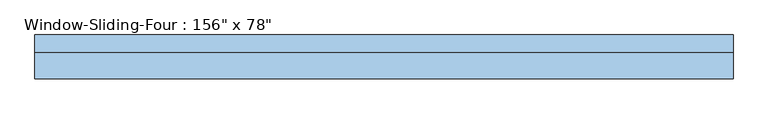
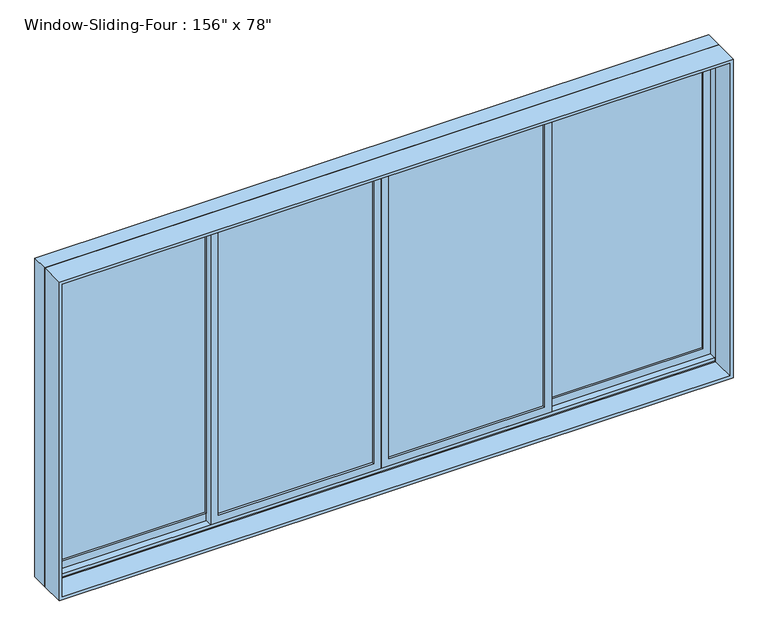
"""IFC4 building model written with IfcOpenShell, lengths in millimetres: window geometry."""

from ifc_helpers import new_model, si_unit, frame, origin, place, context, project, spatial, polyline, outline, extrude, faceted_brep, source, transform, mapped, element, save


def window_8ea0b4a1(model_context):
    return source(origin(), model_context, "Body", "SolidModel", [
        extrude(outline(polyline([(933.45, -1962.15), (933.45, -958.85), (2876.55, -958.85), (2876.55, -1962.15), (933.45, -1962.15)]), holes=[polyline([(2832.1, -1003.3), (996.95, -1003.3), (996.95, -1917.7), (2832.1, -1917.7), (2832.1, -1003.3)])]), frame((0.0, 78.74, 0.0), z_axis=(0.0, 1.0, 0.0), x_axis=(0.0, 0.0, 1.0)), (0.0, 0.0, 1.0), 44.45),
        extrude(outline(polyline([(-1003.3, 110.49), (-1003.3, 104.14), (-1917.7, 104.14), (-1917.7, 110.49), (-1003.3, 110.49)])), frame((0.0, 0.0, 996.95), z_axis=(0.0, 0.0, 1.0), x_axis=(1.0, 0.0, 0.0)), (0.0, 0.0, 1.0), 1835.15),
        extrude(outline(polyline([(-1003.3, 97.79), (-1003.3, 91.44), (-1917.7, 91.44), (-1917.7, 97.79), (-1003.3, 97.79)])), frame((0.0, 0.0, 996.95), z_axis=(0.0, 0.0, 1.0), x_axis=(1.0, 0.0, 0.0)), (0.0, 0.0, 1.0), 1835.15),
        extrude(outline(polyline([(-44.45, 66.04), (-44.45, 59.69), (-958.85, 59.69), (-958.85, 66.04), (-44.45, 66.04)])), frame((0.0, 0.0, 996.95), z_axis=(0.0, 0.0, 1.0), x_axis=(1.0, 0.0, 0.0)), (0.0, 0.0, 1.0), 1835.15),
        extrude(outline(polyline([(-44.45, 53.34), (-44.45, 46.99), (-958.85, 46.99), (-958.85, 53.34), (-44.45, 53.34)])), frame((0.0, 0.0, 996.95), z_axis=(0.0, 0.0, 1.0), x_axis=(1.0, 0.0, 0.0)), (0.0, 0.0, 1.0), 1835.15),
        extrude(outline(polyline([(2895.6, -1981.2), (914.4, -1981.2), (914.4, 1981.2), (2895.6, 1981.2), (2895.6, -1981.2)]), holes=[polyline([(2876.55, 1962.15), (933.45, 1962.15), (933.45, -1962.15), (2876.55, -1962.15), (2876.55, 1962.15)])]), frame((0.0, -118.11, 0.0), z_axis=(0.0, 1.0, 0.0), x_axis=(0.0, 0.0, 1.0)), (0.0, 0.0, 1.0), 146.05),
        extrude(outline(polyline([(952.5, 1003.3), (2876.55, 1003.3), (2876.55, 0.0), (952.5, 0.0), (952.5, 1003.3)]), holes=[polyline([(996.95, 44.45), (2832.1, 44.45), (2832.1, 958.85), (996.95, 958.85), (996.95, 44.45)])]), frame((0.0, 34.29, 0.0), z_axis=(0.0, 1.0, 0.0), x_axis=(0.0, 0.0, 1.0)), (0.0, 0.0, 1.0), 44.45),
        extrude(outline(polyline([(2876.55, -1003.3), (952.5, -1003.3), (952.5, 0.0), (2876.55, 0.0), (2876.55, -1003.3)]), holes=[polyline([(2832.1, -44.45), (996.95, -44.45), (996.95, -958.85), (2832.1, -958.85), (2832.1, -44.45)])]), frame((0.0, 34.29, 0.0), z_axis=(0.0, 1.0, 0.0), x_axis=(0.0, 0.0, 1.0)), (0.0, 0.0, 1.0), 44.45),
        extrude(outline(polyline([(958.85, 66.04), (958.85, 59.69), (44.45, 59.69), (44.45, 66.04), (958.85, 66.04)])), frame((0.0, 0.0, 996.95), z_axis=(0.0, 0.0, 1.0), x_axis=(1.0, 0.0, 0.0)), (0.0, 0.0, 1.0), 1835.15),
        extrude(outline(polyline([(958.85, 53.34), (958.85, 46.99), (44.45, 46.99), (44.45, 53.34), (958.85, 53.34)])), frame((0.0, 0.0, 996.95), z_axis=(0.0, 0.0, 1.0), x_axis=(1.0, 0.0, 0.0)), (0.0, 0.0, 1.0), 1835.15),
        extrude(outline(polyline([(1917.7, 110.49), (1917.7, 104.14), (1003.3, 104.14), (1003.3, 110.49), (1917.7, 110.49)])), frame((0.0, 0.0, 996.95), z_axis=(0.0, 0.0, 1.0), x_axis=(1.0, 0.0, 0.0)), (0.0, 0.0, 1.0), 1835.15),
        extrude(outline(polyline([(1917.7, 97.4725303), (1917.7, 91.44), (1003.3, 91.44), (1003.3, 97.4725303), (1917.7, 97.4725303)])), frame((0.0, 0.0, 996.95), z_axis=(0.0, 0.0, 1.0), x_axis=(1.0, 0.0, 0.0)), (0.0, 0.0, 1.0), 1835.15),
        extrude(outline(polyline([(933.45, 1962.15), (2876.55, 1962.15), (2876.55, 958.85), (933.45, 958.85), (933.45, 1962.15)]), holes=[polyline([(2832.1, 1003.3), (2832.1, 1917.7), (996.95, 1917.7), (996.95, 1003.3), (2832.1, 1003.3)])]), frame((0.0, 78.74, 0.0), z_axis=(0.0, 1.0, 0.0), x_axis=(0.0, 0.0, 1.0)), (0.0, 0.0, 1.0), 44.45),
        faceted_brep([(-1981.2, 27.94, 914.4), (-1981.2, 129.54, 914.4), (1981.2, 129.54, 914.4), (1981.2, 27.94, 914.4), (-1940.2778905, 129.54, 2854.6778905), (-1940.2778905, 123.19, 2854.6778905), (-1940.2778905, 123.19, 933.45), (-1940.2778905, 129.54, 933.45), (1940.2778905, 123.19, 2854.6778905), (1940.2778905, 123.19, 933.45), (1962.15, 123.19, 933.45), (1962.15, 123.19, 2876.55), (-1962.15, 123.19, 2876.55), (-1962.15, 123.19, 933.45), (-1962.15, 27.94, 2876.55), (-1962.15, 27.94, 933.45), (-1962.15, 34.29, 933.45), (-1962.15, 34.29, 952.5), (-1962.15, 78.74, 952.5), (-1962.15, 78.74, 933.45), (1981.2, 27.94, 2895.6), (-1981.2, 27.94, 2895.6), (1962.15, 27.94, 2876.55), (1962.15, 27.94, 933.45), (-1981.2, 129.54, 2895.6), (1981.2, 129.54, 2895.6), (1940.2778905, 129.54, 933.45), (1940.2778905, 129.54, 2854.6778905), (1962.15, 78.74, 933.45), (1962.15, 78.74, 952.5), (1962.15, 34.29, 952.5), (1962.15, 34.29, 933.45)], [[[0, 1, 2, 3]], [[4, 5, 6, 7]], [[5, 8, 9, 10, 11, 12, 13, 6]], [[12, 14, 15, 16, 17, 18, 19, 13]], [[0, 3, 20, 21], [22, 23, 15, 14]], [[24, 1, 0, 21]], [[2, 1, 24, 25], [4, 7, 26, 27]], [[5, 4, 27, 8]], [[12, 11, 22, 14]], [[21, 20, 25, 24]], [[8, 27, 26, 9]], [[22, 11, 10, 28, 29, 30, 31, 23]], [[20, 3, 2, 25]], [[26, 7, 6, 13, 19, 28, 10, 9]], [[28, 19, 18, 29]], [[29, 18, 17, 30]], [[30, 17, 16, 31]], [[15, 23, 31, 16]]]),
    ])


if __name__ == "__main__":
    model = new_model("IFC4")
    model_context = context("Model", 3, world=origin())
    ifc_project = project(units=[si_unit("LENGTHUNIT", "METRE", prefix="MILLI")], contexts=[model_context])
    site = spatial("IfcSite", under=ifc_project)
    building = spatial("IfcBuilding", under=site)
    placement = place(None, origin())
    window_shape = window_8ea0b4a1(model_context)
    element("IfcWindow", 1, ObjectType="Window-Sliding-Four : 156\" x 78\"", at=placement, inside=building, context=model_context, shape_type="MappedRepresentation", body=[
        mapped(window_shape, transform((0.0, 0.0, 0.0), x_axis=(1.0, 0.0, 0.0), y_axis=(0.0, 1.0, 0.0), z_axis=(0.0, 0.0, 1.0))),
    ])
    save(model, "model.ifc")

# Revit data of these elements
# Type "Window-Sliding-Four : 156\" x 78\""
#   Type Mark = "21"
#   Fire Rating = "0.5h"
#   Assembly Code = "B2020100"
#   Analytic Construction = "Double glazing - domestic"
#   Window Inset [instance default] = 0 ft
#   Wall Thickness [instance default] = 0.5 ft
#   Visual Light Transmittance = 0.81
#   Thermal Resistance (R) = 1.8146 (h·ft²·°F)/BTU
#   Solar Heat Gain Coefficient = 0.76
#   Interior Wall Closure [instance default] = 0.216146 ft
#   Heat Transfer Coefficient (U) = 0.5511 BTU/(h·ft²·°F)
#   Frame Extension [instance default] = 0.020833 ft
#   Exterior Wall Closure [instance default] = 0.104167 ft
#   Rough Width = 13.041667 ft
#   Rough Height = 6.541667 ft
#   Height = 6.5 ft
#   Extension Jamb [instance default] = 0.229167 ft
#   Default Sill Height = 3 ft
#   Width = 13 ft
#   Middle Muntin Visibility = yes
#   Interior Trim Visibility [instance default] = yes
#   Indicator Visibility [instance default] = yes
#   Exterior Trim Visibility [instance default] = yes
#   Side Muntin Visibility = yes
#   Extension Jamb Visibility [instance default] = yes
#   Interior Trim Material = Wood - Stained
#   Muntin Pattern = Muntin Pattern_2x2 : Muntin Pattern_2x2
#   Interior Trim = Trim-Window-Interior-Flat : Picture Frame
#   Interior Frame Material = Wood - Stained
#   Glass Panel Material = Glass
#   Exterior Trim Material = Clad - White
#   Exterior Trim = Trim-Window-Exterior-Flat : with Sill
#   Exterior Frame Material = Clad - White
#   Wall Closure = (empty or 0)
# Element 1 (IfcWindow, "Window-Sliding-Four : 156\" x 78\"")
#   Wall Thickness = 0.75 ft
#   Extension Jamb = 0.479167 ft
#   Materials on its faces: "Wood - Stained", "Glass", "Clad - White"
# Materials
#   "Wood - Stained": class "Wood", colour RGB 224 178 126, transparency 0, Cost = 0
#   "Glass": class "Glass", colour RGB 0 128 192, transparency 0.75, Description = "Soda Lime Glass", Cost = 0
#   "Clad - White": class "Wood", colour RGB 242 242 238, transparency 0, Cost = 0
